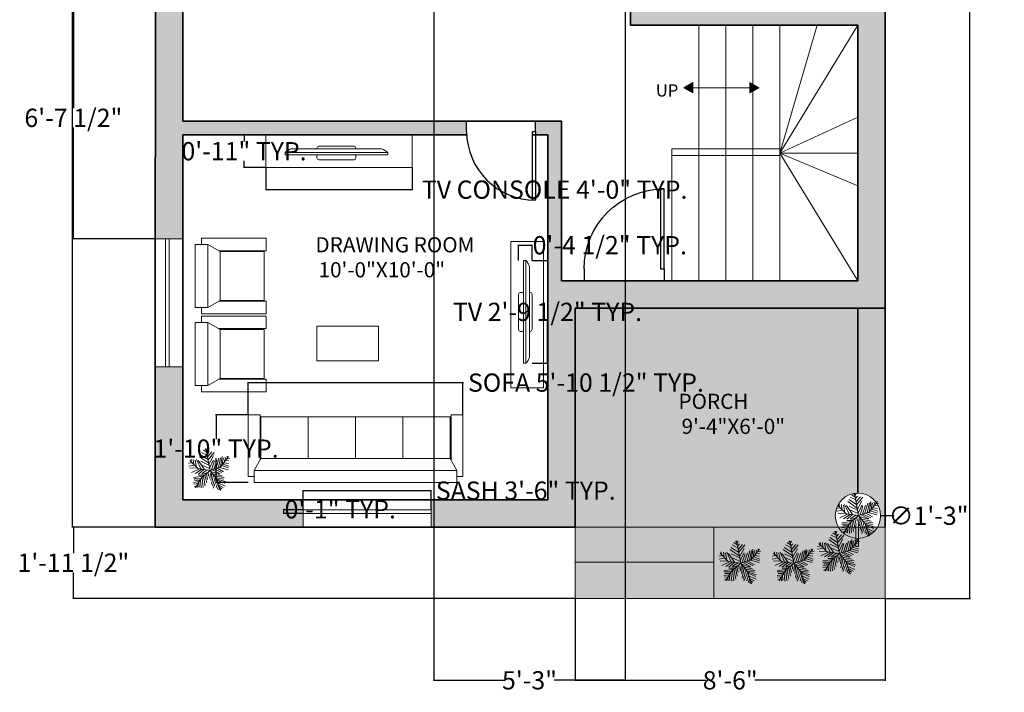
# Model space of a CAD drawing. Units: inches. Extents: x 143233372 to 143233714, y 112671713 to 112672292.
# Tile 1 of 7: x 143233372 to 143233695, y 112671713 to 112671935. Entities that reach past the tile are written whole.
import ezdxf

# ---------------------------------------------------------------- set-up
doc = ezdxf.new("R2010")
doc.units = ezdxf.units.IN
doc.header["$MEASUREMENT"] = 0
doc.layers.get('0').update_dxf_attribs({"color": 104})
for name, color, linetype, lineweight in [('A-ANNO-DIMS', 2, 'Continuous', 18), ('A-ANNO-SYMB', 7, 'Continuous', 18), ('A-AREA-IDEN', 7, 'Continuous', 18), ('A-EQPM', 8, 'Continuous', 18), ('A-FLOR-STRS', 7, 'Continuous', 18), ('doors', 32, 'Continuous', 25), ('furniture', 23, 'Continuous', 18), ('L-PLNT', 92, 'Continuous', 13), ('L-PLNT-BEDS', 94, 'Continuous', 18), ('L-PLNT-PATT', 92, 'Continuous', 9), ('text', 7, 'Continuous', 18), ('walls', 7, 'Continuous', 35), ('windows', 4, 'Continuous', 18)]:
    doc.layers.add(name, color=color, linetype=linetype, lineweight=lineweight)
doc.layers.add('A-FLOR-PATT', color=9, linetype='Continuous', lineweight=9, true_color=0xc7c8ca)
doc.layers.add('A-WALL-PATT', color=18, linetype='Continuous', lineweight=9, true_color=0x000000)
doc.styles.get("Standard").update_dxf_attribs({"font": 'arial.ttf'})
doc.dimstyles.get("Standard").update_dxf_attribs({"dimtxt": 6, "dimasz": 0.18, "dimexe": 0.18, "dimexo": 0.0625, "dimgap": 0.09, "dimtad": 0, "dimtih": 1, "dimtoh": 1, "dimzin": 0, "dimdsep": 46, "dimlunit": 3, "dimtxsty": 'Standard', "dimcen": 0.09, "dimadec": 0, "dimazin": 0, "dimtfac": 1, "dimtofl": 0, "dimtmove": 0, "dimatfit": 3, "dimfxl": 1, "dimtolj": 1, "dimtzin": 0, "dimarcsym": 0})

# ---------------------------------------------------------------- blocks, each defined once
blk = doc.blocks.new('FABRIC SOFA 4S')
at = {"layer": 'furniture'}
for p, q in [((0, -51), (0, 51)), ((6, 51), (0, 51)), ((3, 54), (34, 54)), ((3, 51), (3, 54)), ((6, -51), (6, 51)), ((12, 47.63), (6, 51)), ((34, 48), (34, 54)), ((11.14, 48), (34, 48)), ((33, 23.81), (12, 23.81)), ((33, 0), (12, 0)), ((33, -23.81), (12, -23.81)), ((6, -51), (12, -47.63)), ((11.54, -48), (34, -48)), ((34, -48), (34, -54)), ((6, -51), (0, -51)), ((3, -54), (3, -51)), ((3, -54), (34, -54))]:
    blk.add_line(p, q, dxfattribs=at)
blk.add_lwpolyline([(12, -47.63), (12, 47.63), (33, 47.63), (33, -47.63)], close=True, dxfattribs=at)
blk = doc.blocks.new('FABRIC SOFA 1S')
at = {"layer": 'furniture'}
for p, q in [((0, -15.12), (0, 15.12)), ((6, 15.12), (0, 15.12)), ((3, 18.12), (34, 18.12)), ((3, 15.12), (3, 18.12)), ((6, -15.12), (6, 15.12)), ((12, 11.75), (6, 15.12)), ((34, 12.12), (34, 18.12)), ((11.33, 12.12), (34, 12.12)), ((6, -15.12), (12, -11.75)), ((11.33, -12.12), (34, -12.12)), ((34, -12.12), (34, -18.12)), ((6, -15.12), (0, -15.12)), ((3, -18.12), (3, -15.12)), ((3, -18.12), (34, -18.12))]:
    blk.add_line(p, q, dxfattribs=at)
blk.add_lwpolyline([(12, -11.75), (12, 11.75), (33, 11.75), (33, -11.75)], close=True, dxfattribs=at)
blk = doc.blocks.new('PLASMA-LARGE')
at = {"layer": 'furniture'}
for p, q in [((-7.26, 0), (7.26, 0)), ((-21, -2.5), (21, -2.5)), ((-21, -2.5), (-21, -3.5)), ((-21, -3.5), (21, -3.5)), ((-18.61, -1), (18.61, -1)), ((-8, -1), (-8, -0.74)), ((-8, -3.5), (-8, -4.76)), ((8, -1), (8, -0.74)), ((8, -3.5), (8, -4.76)), ((21, -2.5), (21, -3.5)), ((-7.26, -5.5), (7.26, -5.5))]:
    blk.add_line(p, q, dxfattribs=at)
for centre, radius, start, end in [((-7.26, -0.74), 0.744, 90, 180), ((7.26, -0.74), 0.744, 0, 90), ((-13.97, -11.05), 11.07, 114.7602, 129.4175), ((13.97, -11.05), 11.07, 50.5825, 65.2398), ((-7.26, -4.76), 0.744, 180, 270), ((7.26, -4.76), 0.744, 270, 0)]:
    blk.add_arc(centre, radius, start, end, dxfattribs=at)
blk = doc.blocks.new('*U24')
for p, q in [((0, 0), (0, -6)), ((40, 0), (40, -6))]:
    blk.add_line(p, q)
blk.add_lwpolyline([(0, 0), (0, 40), (1.75, 40), (1.75, 0)], close=True)
blk.add_arc((0, 0), 40, 0, 90)
blk = doc.blocks.new('*U26')
for p, q in [((-8.737, 47.138), (-17.069, 52.711)), ((-10.186, 53.64), (-13.084, 55.962)), ((0, 0), (-10.5, 57)), ((-9.099, 51.782), (-6.563, 55.962)), ((-31.5, 4.5), (-52.5, 25.5)), ((-48.585, 21.131), (-49.309, 29.026)), ((-43.513, 28.561), (-42.427, 15.558)), ((-38.442, 26.239), (-34.819, 7.663)), ((-35.544, 28.097), (-24.314, 3.947)), ((-14.533, 2.09), (-30.834, 25.31)), ((-3.665, 19.273), (-27.574, 35.527)), ((-5.114, 28.097), (-24.676, 40.636)), ((-7.288, 39.707), (-21.778, 46.673)), ((-7.65, 43.423), (-2.578, 49.46)), ((-5.839, 35.992), (4.667, 48.067)), ((-5.114, 27.632), (10.463, 46.673)), ((-2.941, 16.486), (8.652, 37.85)), ((-1.129, 6.734), (9.014, 26.704)), ((10.101, 3.483), (17.708, 26.239)), ((16.259, 5.805), (23.142, 31.348)), ((22.055, 7.198), (27.489, 32.277)), ((27, 9), (48, 36)), ((27.127, 9.056), (31.112, 35.992)), ((31.836, 30.883), (32.561, 16.486)), ((35.096, 32.741), (37.27, 22.524)), ((38.719, 34.134), (41.979, 28.561)), ((40.53, 25.775), (48.862, 24.846)), ((43.791, 29.954), (51.036, 30.883)), ((44.153, 36.456), (45.239, 32.741)), ((-47.498, 19.737), (-55.83, 18.344)), ((-40.615, 13.7), (-55.105, 10.913)), ((-33.37, 6.269), (-52.207, 5.34)), ((-28.299, 3.483), (-47.86, -5.805)), ((-21.416, 3.018), (-38.079, -8.128)), ((0, 0), (-31.5, 4.5)), ((-15.982, 2.09), (-30.11, -9.521)), ((-24.314, 23.917), (-2.941, 13.7)), ((0, 0), (-22.5, -19.5)), ((-6.563, 1.161), (-21.416, -8.128)), ((-20.691, 13.7), (-1.129, 4.876)), ((0, 0), (27, 9)), ((0, 0), (18, -22.5)), ((3.942, 1.625), (11.187, 24.381)), ((6.478, 1.625), (26.04, -8.592)), ((11.187, 3.483), (30.749, -5.805)), ((18.07, 5.805), (35.096, -3.483)), ((24.229, 7.663), (46.688, 1.625)), ((29.662, 12.307), (48.137, 6.269)), ((33.285, 16.486), (48.862, 10.913)), ((36.183, 19.737), (48.137, 17.88)), ((-17.431, -15.094), (-42.789, -18.809)), ((-24.314, -21.596), (-42.427, -22.06)), ((-22.5, -19.5), (-37.5, -45)), ((-15.257, -12.772), (-30.11, -12.772)), ((-25.038, -23.918), (-22.865, -45.281)), ((-20.691, -18.345), (-17.793, -44.352)), ((-6.563, -5.805), (-19.967, -9.985)), ((-17.069, -15.094), (-12.721, -40.172)), ((-13.446, -11.378), (-8.737, -32.741)), ((-9.461, -8.592), (-6.201, -23.453)), ((-4.752, -3.483), (-3.665, -14.629)), ((2.493, -3.019), (-1.491, -20.202)), ((1.769, -2.555), (24.229, -9.521)), ((5.029, -6.27), (2.131, -25.775)), ((9.014, -11.378), (3.58, -35.992)), ((14.085, -16.951), (6.478, -40.172)), ((7.565, -9.056), (32.198, -14.629)), ((18.07, -22.524), (8.289, -45.745)), ((12.274, -15.094), (36.907, -18.809)), ((16.259, -19.738), (36.183, -22.989)), ((18, -22.5), (27, -52.5)), ((18.433, -22.524), (40.53, -29.026)), ((-28.299, -29.026), (-42.789, -31.348)), ((-30.834, -34.135), (-42.427, -35.528)), ((-34.457, -39.708), (-40.978, -42.494)), ((-26.849, -26.24), (-40.253, -25.775)), ((-32.646, -36.921), (-31.921, -44.352)), ((-29.023, -30.884), (-27.936, -43.887)), ((20.244, -30.419), (15.897, -44.816)), ((19.157, -25.311), (38.719, -33.206)), ((22.78, -37.85), (19.519, -48.532)), ((21.331, -32.741), (39.081, -40.636)), ((22.78, -38.314), (34.372, -44.816)), ((24.591, -45.745), (23.142, -50.854)), ((24.591, -43.423), (30.749, -47.603)), ((26.764, -49.925), (28.213, -50.854))]:
    blk.add_line(p, q)
blk = doc.blocks.new('*D28')
at = {"layer": 'A-ANNO-DIMS', "color": 0, "lineweight": -2, "transparency": 16777216}
for p, q in [((143233416.22, 112672249.18), (143233388.75, 112672249.18)), ((143233388.93, 112672249), (143233388.93, 112672011.59)), ((143233388.93, 112671767.86), (143233388.93, 112672005.28)), ((143233416.22, 112671767.68), (143233388.75, 112671767.68))]:
    blk.add_line(p, q, dxfattribs=at)
at = {"layer": 'A-ANNO-DIMS', "color": 0, "transparency": 16777216}
for points in [[(143233388.9, 112672249), (143233388.96, 112672249), (143233388.93, 112672249.18)], [(143233388.9, 112671767.86), (143233388.96, 112671767.86), (143233388.93, 112671767.68)]]:
    blk.add_solid(points, dxfattribs=at)
at = {"layer": 'Defpoints', "color": 0, "transparency": 16777216}
for p in [(143233416.28, 112672249.18), (143233388.93, 112671767.68), (143233416.28, 112671767.68)]:
    blk.add_point(p, dxfattribs=at)
at = {"layer": 'A-ANNO-DIMS', "color": 0, "transparency": 16777216, "insert": (143233388.93, 112672008.43), "char_height": 6, "attachment_point": 5}
blk.add_mtext('\\A1;30\'-0"', dxfattribs=at)
blk = doc.blocks.new('SASH-42IN')
for p, q in [((0, 1.17), (42.12, 1.17)), ((42.12, 0), (0, 0)), ((42.12, 1.17), (42.12, 0))]:
    blk.add_line(p, q)
blk = doc.blocks.new('MEDIA-CONSOLE')
for p, q in [((0, 48.12), (10.82, 48.12)), ((0, 0), (0, 48.12)), ((10.82, 48.12), (10.82, 0)), ((10.82, 0), (0, 0))]:
    blk.add_line(p, q)
blk = doc.blocks.new('*D33')
at = {"layer": 'A-ANNO-DIMS', "color": 0, "lineweight": -2, "transparency": 16777216}
for p, q in [((143233464.81, 112671773.41), (143233464.81, 112671779.85)), ((143233464.99, 112671779.67), (143233506.74, 112671779.67)), ((143233506.92, 112671773.41), (143233506.92, 112671779.85)), ((143233506.92, 112671779.67), (143233507.1, 112671779.67))]:
    blk.add_line(p, q, dxfattribs=at)
at = {"layer": 'A-ANNO-DIMS', "color": 0, "transparency": 16777216}
for points in [[(143233464.99, 112671779.7), (143233464.99, 112671779.64), (143233464.81, 112671779.67)], [(143233506.74, 112671779.7), (143233506.74, 112671779.64), (143233506.92, 112671779.67)]]:
    blk.add_solid(points, dxfattribs=at)
at = {"layer": 'Defpoints', "color": 0, "transparency": 16777216}
for p in [(143233506.92, 112671779.67), (143233464.81, 112671773.35), (143233506.92, 112671773.35)]:
    blk.add_point(p, dxfattribs=at)
at = {"layer": 'A-ANNO-DIMS', "color": 0, "transparency": 16777216, "insert": (143233538.04, 112671779.67), "char_height": 6, "attachment_point": 5}
blk.add_mtext('\\A1;SASH 3\'-6" TYP.', dxfattribs=at)
blk = doc.blocks.new('*D34')
at = {"layer": 'A-ANNO-DIMS', "color": 0, "lineweight": -2, "transparency": 16777216}
for p, q in [((143233464.74, 112671773.35), (143233458.31, 112671773.35)), ((143233464.74, 112671772.18), (143233458.31, 112671772.18)), ((143233458.49, 112671773.35), (143233458.49, 112671773.53)), ((143233458.49, 112671773.53), (143233458.67, 112671773.53)), ((143233458.49, 112671772.36), (143233458.49, 112671773.17))]:
    blk.add_line(p, q, dxfattribs=at)
at = {"layer": 'A-ANNO-DIMS', "color": 0, "transparency": 16777216}
for points in [[(143233458.46, 112671773.17), (143233458.52, 112671773.17), (143233458.49, 112671773.35)], [(143233458.46, 112671772.36), (143233458.52, 112671772.36), (143233458.49, 112671772.18)]]:
    blk.add_solid(points, dxfattribs=at)
at = {"layer": 'Defpoints', "color": 0, "transparency": 16777216}
for p in [(143233458.49, 112671773.35), (143233464.81, 112671773.35), (143233464.81, 112671772.18)]:
    blk.add_point(p, dxfattribs=at)
at = {"layer": 'A-ANNO-DIMS', "color": 0, "transparency": 16777216, "insert": (143233477.04, 112671773.53), "char_height": 6, "attachment_point": 5}
blk.add_mtext('\\A1;0\'-1" TYP.', dxfattribs=at)
blk = doc.blocks.new('*D37')
at = {"layer": 'A-ANNO-DIMS', "color": 0, "lineweight": -2, "transparency": 16777216}
for p, q in [((143233540.19, 112671855.3), (143233545.37, 112671855.3)), ((143233545.19, 112671855.12), (143233545.19, 112671841.63)), ((143233545.19, 112671821.75), (143233545.19, 112671835.24)), ((143233540.19, 112671821.57), (143233545.37, 112671821.57))]:
    blk.add_line(p, q, dxfattribs=at)
at = {"layer": 'A-ANNO-DIMS', "color": 0, "transparency": 16777216}
for points in [[(143233545.16, 112671855.12), (143233545.22, 112671855.12), (143233545.19, 112671855.3)], [(143233545.16, 112671821.75), (143233545.22, 112671821.75), (143233545.19, 112671821.57)]]:
    blk.add_solid(points, dxfattribs=at)
at = {"layer": 'Defpoints', "color": 0, "transparency": 16777216}
for p in [(143233540.13, 112671855.3), (143233540.13, 112671821.57), (143233545.19, 112671821.57)]:
    blk.add_point(p, dxfattribs=at)
at = {"layer": 'A-ANNO-DIMS', "color": 0, "transparency": 16777216, "insert": (143233545.19, 112671838.44), "char_height": 6, "attachment_point": 5}
blk.add_mtext('\\A1;TV 2\'-9 1/2" TYP.', dxfattribs=at)
blk = doc.blocks.new('*D38')
at = {"layer": 'A-ANNO-DIMS', "color": 0, "lineweight": -2, "transparency": 16777216}
for p, q in [((143233535.71, 112671855.36), (143233535.71, 112671860.54)), ((143233535.89, 112671860.36), (143233539.95, 112671860.36)), ((143233540.13, 112671855.36), (143233540.13, 112671860.54)), ((143233540.13, 112671860.36), (143233540.31, 112671860.36))]:
    blk.add_line(p, q, dxfattribs=at)
at = {"layer": 'A-ANNO-DIMS', "color": 0, "transparency": 16777216}
for points in [[(143233535.89, 112671860.39), (143233535.89, 112671860.33), (143233535.71, 112671860.36)], [(143233539.95, 112671860.39), (143233539.95, 112671860.33), (143233540.13, 112671860.36)]]:
    blk.add_solid(points, dxfattribs=at)
at = {"layer": 'Defpoints', "color": 0, "transparency": 16777216}
for p in [(143233540.13, 112671860.36), (143233535.71, 112671855.3), (143233540.13, 112671855.3)]:
    blk.add_point(p, dxfattribs=at)
at = {"layer": 'A-ANNO-DIMS', "color": 0, "transparency": 16777216, "insert": (143233565.68, 112671860.36), "char_height": 6, "attachment_point": 5}
blk.add_mtext('\\A1;0\'-4 1/2" TYP.', dxfattribs=at)
blk = doc.blocks.new('*D39')
at = {"layer": 'A-ANNO-DIMS', "color": 0, "lineweight": -2, "transparency": 16777216}
for p, q in [((143233452.61, 112671885.8), (143233452.61, 112671878.46)), ((143233500.73, 112671885.8), (143233500.73, 112671878.46)), ((143233452.79, 112671878.64), (143233500.55, 112671878.64)), ((143233500.73, 112671878.64), (143233500.91, 112671878.64))]:
    blk.add_line(p, q, dxfattribs=at)
at = {"layer": 'A-ANNO-DIMS', "color": 0, "transparency": 16777216}
for points in [[(143233452.79, 112671878.67), (143233452.79, 112671878.61), (143233452.61, 112671878.64)], [(143233500.55, 112671878.67), (143233500.55, 112671878.61), (143233500.73, 112671878.64)]]:
    blk.add_solid(points, dxfattribs=at)
at = {"layer": 'Defpoints', "color": 0, "transparency": 16777216}
for p in [(143233452.61, 112671885.86), (143233500.73, 112671885.86), (143233500.73, 112671878.64)]:
    blk.add_point(p, dxfattribs=at)
at = {"layer": 'A-ANNO-DIMS', "color": 0, "transparency": 16777216, "insert": (143233547.54, 112671878.64), "char_height": 6, "attachment_point": 5}
blk.add_mtext('\\A1;TV CONSOLE 4\'-0" TYP.', dxfattribs=at)
blk = doc.blocks.new('*D40')
at = {"layer": 'A-ANNO-DIMS', "color": 0, "lineweight": -2, "transparency": 16777216}
for p, q in [((143233452.55, 112671896.68), (143233445.21, 112671896.68)), ((143233445.39, 112671896.5), (143233445.39, 112671894.42)), ((143233445.39, 112671886.04), (143233445.39, 112671888.12)), ((143233452.55, 112671885.86), (143233445.21, 112671885.86))]:
    blk.add_line(p, q, dxfattribs=at)
at = {"layer": 'A-ANNO-DIMS', "color": 0, "transparency": 16777216}
for points in [[(143233445.36, 112671896.5), (143233445.42, 112671896.5), (143233445.39, 112671896.68)], [(143233445.36, 112671886.04), (143233445.42, 112671886.04), (143233445.39, 112671885.86)]]:
    blk.add_solid(points, dxfattribs=at)
at = {"layer": 'Defpoints', "color": 0, "transparency": 16777216}
for p in [(143233452.61, 112671896.68), (143233445.39, 112671885.86), (143233452.61, 112671885.86)]:
    blk.add_point(p, dxfattribs=at)
at = {"layer": 'A-ANNO-DIMS', "color": 0, "transparency": 16777216, "insert": (143233445.39, 112671891.27), "char_height": 6, "attachment_point": 5}
blk.add_mtext('\\A1;0\'-11" TYP.', dxfattribs=at)
blk = doc.blocks.new('*D45')
at = {"layer": 'A-ANNO-DIMS', "color": 0, "lineweight": -2, "transparency": 16777216}
for p, q in [((143233446.78, 112671804.66), (143233446.78, 112671815.37)), ((143233446.96, 112671815.19), (143233517.21, 112671815.19)), ((143233517.39, 112671804.66), (143233517.39, 112671815.37)), ((143233517.39, 112671815.19), (143233517.57, 112671815.19))]:
    blk.add_line(p, q, dxfattribs=at)
at = {"layer": 'A-ANNO-DIMS', "color": 0, "transparency": 16777216}
for points in [[(143233446.96, 112671815.22), (143233446.96, 112671815.16), (143233446.78, 112671815.19)], [(143233517.21, 112671815.22), (143233517.21, 112671815.16), (143233517.39, 112671815.19)]]:
    blk.add_solid(points, dxfattribs=at)
at = {"layer": 'Defpoints', "color": 0, "transparency": 16777216}
for p in [(143233517.39, 112671815.19), (143233446.78, 112671804.6), (143233517.39, 112671804.6)]:
    blk.add_point(p, dxfattribs=at)
at = {"layer": 'A-ANNO-DIMS', "color": 0, "transparency": 16777216, "insert": (143233557.83, 112671815.19), "char_height": 6, "attachment_point": 5}
blk.add_mtext('\\A1;SOFA 5\'-10 1/2" TYP.', dxfattribs=at)
blk = doc.blocks.new('*D46')
at = {"layer": 'A-ANNO-DIMS', "color": 0, "lineweight": -2, "transparency": 16777216}
for p, q in [((143233446.71, 112671804.6), (143233436.01, 112671804.6)), ((143233436.19, 112671804.42), (143233436.19, 112671796.64)), ((143233436.19, 112671782.55), (143233436.19, 112671790.33)), ((143233446.71, 112671782.37), (143233436.01, 112671782.37))]:
    blk.add_line(p, q, dxfattribs=at)
at = {"layer": 'A-ANNO-DIMS', "color": 0, "transparency": 16777216}
for points in [[(143233436.16, 112671804.42), (143233436.22, 112671804.42), (143233436.19, 112671804.6)], [(143233436.16, 112671782.55), (143233436.22, 112671782.55), (143233436.19, 112671782.37)]]:
    blk.add_solid(points, dxfattribs=at)
at = {"layer": 'Defpoints', "color": 0, "transparency": 16777216}
for p in [(143233436.19, 112671804.6), (143233446.78, 112671804.6), (143233446.78, 112671782.37)]:
    blk.add_point(p, dxfattribs=at)
at = {"layer": 'A-ANNO-DIMS', "color": 0, "transparency": 16777216, "insert": (143233436.19, 112671793.49), "char_height": 6, "attachment_point": 5}
blk.add_mtext('\\A1;1\'-10" TYP.', dxfattribs=at)
blk = doc.blocks.new('*D63')
at = {"layer": 'A-ANNO-DIMS', "color": 0, "lineweight": -2, "transparency": 16777216}
for p, q in [((143233656.35, 112672249.18), (143233684.29, 112672249.18)), ((143233684.11, 112672249), (143233684.11, 112671999.82)), ((143233684.11, 112671744.43), (143233684.11, 112671993.61)), ((143233656.35, 112671744.25), (143233684.29, 112671744.25))]:
    blk.add_line(p, q, dxfattribs=at)
at = {"layer": 'A-ANNO-DIMS', "color": 0, "transparency": 16777216}
for points in [[(143233684.08, 112672249), (143233684.14, 112672249), (143233684.11, 112672249.18)], [(143233684.08, 112671744.43), (143233684.14, 112671744.43), (143233684.11, 112671744.25)]]:
    blk.add_solid(points, dxfattribs=at)
at = {"layer": 'Defpoints', "color": 0, "transparency": 16777216}
for p in [(143233656.28, 112672249.18), (143233656.28, 112671744.25), (143233684.11, 112671744.25)]:
    blk.add_point(p, dxfattribs=at)
at = {"layer": 'A-ANNO-DIMS', "color": 0, "transparency": 16777216, "insert": (143233684.11, 112671996.72), "char_height": 6, "attachment_point": 5}
blk.add_mtext('\\A1;42\'-1"', dxfattribs=at)
blk = doc.blocks.new('*D67')
at = {"layer": 'A-ANNO-DIMS', "color": 0, "lineweight": -2, "transparency": 16777216}
for p, q in [((143233554.28, 112671744.19), (143233554.28, 112671717.12)), ((143233656.28, 112671744.19), (143233656.28, 112671717.12)), ((143233554.46, 112671717.3), (143233597.22, 112671717.3)), ((143233656.1, 112671717.3), (143233613.35, 112671717.3))]:
    blk.add_line(p, q, dxfattribs=at)
at = {"layer": 'A-ANNO-DIMS', "color": 0, "transparency": 16777216}
for points in [[(143233554.46, 112671717.33), (143233554.46, 112671717.27), (143233554.28, 112671717.3)], [(143233656.1, 112671717.33), (143233656.1, 112671717.27), (143233656.28, 112671717.3)]]:
    blk.add_solid(points, dxfattribs=at)
at = {"layer": 'Defpoints', "color": 0, "transparency": 16777216}
for p in [(143233554.28, 112671744.25), (143233656.28, 112671744.25), (143233554.28, 112671717.3)]:
    blk.add_point(p, dxfattribs=at)
at = {"layer": 'A-ANNO-DIMS', "color": 0, "transparency": 16777216, "insert": (143233605.28, 112671717.3), "char_height": 6, "attachment_point": 5}
blk.add_mtext('\\A1;8\'-6"', dxfattribs=at)
blk = doc.blocks.new('*D68')
at = {"layer": 'A-ANNO-DIMS', "color": 0, "lineweight": -2, "transparency": 16777216}
for p, q in [((143233554.22, 112671767.68), (143233389.09, 112671767.68)), ((143233389.27, 112671767.5), (143233389.27, 112671759.16)), ((143233389.27, 112671744.43), (143233389.27, 112671752.77)), ((143233554.22, 112671744.25), (143233389.09, 112671744.25))]:
    blk.add_line(p, q, dxfattribs=at)
at = {"layer": 'A-ANNO-DIMS', "color": 0, "transparency": 16777216}
for points in [[(143233389.24, 112671767.5), (143233389.3, 112671767.5), (143233389.27, 112671767.68)], [(143233389.24, 112671744.43), (143233389.3, 112671744.43), (143233389.27, 112671744.25)]]:
    blk.add_solid(points, dxfattribs=at)
at = {"layer": 'Defpoints', "color": 0, "transparency": 16777216}
for p in [(143233389.27, 112671767.68), (143233554.28, 112671767.68), (143233554.28, 112671744.25)]:
    blk.add_point(p, dxfattribs=at)
at = {"layer": 'A-ANNO-DIMS', "color": 0, "transparency": 16777216, "insert": (143233389.27, 112671755.97), "char_height": 6, "attachment_point": 5}
blk.add_mtext('\\A1;1\'-11 1/2"', dxfattribs=at)
blk = doc.blocks.new('*D69')
at = {"layer": 'A-ANNO-DIMS', "color": 0, "lineweight": -2, "transparency": 16777216}
for p, q in [((143233507.78, 112672033.12), (143233507.78, 112671717.12)), ((143233570.78, 112672033.12), (143233570.78, 112671717.12)), ((143233507.96, 112671717.3), (143233531.22, 112671717.3)), ((143233570.6, 112671717.3), (143233547.35, 112671717.3))]:
    blk.add_line(p, q, dxfattribs=at)
at = {"layer": 'A-ANNO-DIMS', "color": 0, "transparency": 16777216}
for points in [[(143233507.96, 112671717.33), (143233507.96, 112671717.27), (143233507.78, 112671717.3)], [(143233570.6, 112671717.33), (143233570.6, 112671717.27), (143233570.78, 112671717.3)]]:
    blk.add_solid(points, dxfattribs=at)
at = {"layer": 'Defpoints', "color": 0, "transparency": 16777216}
for p in [(143233507.78, 112672033.18), (143233570.78, 112672033.18), (143233570.78, 112671717.3)]:
    blk.add_point(p, dxfattribs=at)
at = {"layer": 'A-ANNO-DIMS', "color": 0, "transparency": 16777216, "insert": (143233539.28, 112671717.3), "char_height": 6, "attachment_point": 5}
blk.add_mtext('\\A1;5\'-3"', dxfattribs=at)
blk = doc.blocks.new('*D73')
at = {"layer": 'A-ANNO-DIMS', "color": 0, "lineweight": -2, "transparency": 16777216}
for p, q in [((143233416.22, 112671942.04), (143233389.09, 112671942.04)), ((143233389.27, 112671941.86), (143233389.27, 112671905.44)), ((143233389.27, 112671862.63), (143233389.27, 112671899.05)), ((143233416.22, 112671862.45), (143233389.09, 112671862.45))]:
    blk.add_line(p, q, dxfattribs=at)
at = {"layer": 'A-ANNO-DIMS', "color": 0, "transparency": 16777216}
for points in [[(143233389.24, 112671941.86), (143233389.3, 112671941.86), (143233389.27, 112671942.04)], [(143233389.24, 112671862.63), (143233389.3, 112671862.63), (143233389.27, 112671862.45)]]:
    blk.add_solid(points, dxfattribs=at)
at = {"layer": 'Defpoints', "color": 0, "transparency": 16777216}
for p in [(143233389.27, 112671942.04), (143233416.28, 112671942.04), (143233416.28, 112671862.45)]:
    blk.add_point(p, dxfattribs=at)
at = {"layer": 'A-ANNO-DIMS', "color": 0, "transparency": 16777216, "insert": (143233389.27, 112671902.24), "char_height": 6, "attachment_point": 5}
blk.add_mtext('\\A1;6\'-7 1/2"', dxfattribs=at)
blk = doc.blocks.new('*D78')
at = {"layer": 'A-ANNO-DIMS', "color": 0, "lineweight": -2, "transparency": 16777216}
for p, q in [((143233647.19, 112671771.42), (143233647.37, 112671771.42)), ((143233647.28, 112671771.33), (143233647.28, 112671771.51)), ((143233659.18, 112671771.42), (143233654.9, 112671771.42))]:
    blk.add_line(p, q, dxfattribs=at)
at = {"layer": 'A-ANNO-DIMS', "color": 0, "transparency": 16777216}
blk.add_solid([(143233654.9, 112671771.45), (143233654.9, 112671771.39), (143233654.72, 112671771.42)], dxfattribs=at)
at = {"layer": 'Defpoints', "color": 0, "transparency": 16777216}
for p in [(143233639.85, 112671771.42), (143233654.72, 112671771.42)]:
    blk.add_point(p, dxfattribs=at)
at = {"layer": 'A-ANNO-DIMS', "color": 0, "transparency": 16777216, "insert": (143233670.51, 112671771.42), "char_height": 6, "attachment_point": 5}
blk.add_mtext('\\A1;∅1\'-3"', dxfattribs=at)

msp = doc.modelspace()

# ---------------------------------------------------------------- hatches: boundary and pattern name
at = {"layer": 'A-ANNO-SYMB'}
h = msp.add_hatch(color=256, dxfattribs=at)
h.dxf.hatch_style = 1
h.paths.add_polyline_path([(143233593.014, 112671913.81), (143233589.979, 112671912.056), (143233593.014, 112671910.417)])
h = msp.add_hatch(color=256, dxfattribs=at)
h.dxf.hatch_style = 1
h.paths.add_polyline_path([(143233611.75, 112671910.417), (143233614.785, 112671912.056), (143233611.75, 112671913.81)])
at = {"layer": 'A-FLOR-PATT'}
h = msp.add_hatch(color=256, dxfattribs=at)
h.dxf.hatch_style = 1
h.paths.add_polyline_path([(143233647.285, 112671839.682), (143233554.285, 112671839.682), (143233554.285, 112671767.682), (143233599.887, 112671767.682), (143233640.858, 112671767.682, -0.1325091), (143233639.849, 112671771.421, -0.4142136), (143233647.285, 112671778.857)])
h.paths.add_polyline_path([(143233656.285, 112671839.682), (143233647.285, 112671839.682), (143233647.285, 112671778.857, -0.4142136), (143233654.72, 112671771.421, -0.1325091), (143233653.711, 112671767.682), (143233656.285, 112671767.682)])
h.paths.add_polyline_path([(143233599.887, 112671767.682), (143233599.887, 112671767.682), (143233554.285, 112671767.682), (143233554.285, 112671756.172), (143233599.887, 112671756.172)])
h.paths.add_polyline_path([(143233599.887, 112671756.172), (143233554.285, 112671756.172), (143233554.285, 112671744.249), (143233599.887, 112671744.249)])
at = {"layer": 'A-WALL-PATT'}
h = msp.add_hatch(color=256, dxfattribs=at)
h.dxf.hatch_style = 1
h.paths.add_polyline_path([(143233425.285, 112671820.328), (143233416.222, 112671820.328), (143233416.222, 112671767.682), (143233464.805, 112671767.682), (143233464.805, 112671776.682), (143233425.285, 112671776.682)])
h.paths.add_polyline_path([(143233425.285, 112672055.48), (143233416.285, 112672055.48), (143233416.285, 112671984.159), (143233425.285, 112671984.159)])
h.paths.add_polyline_path([(143233656.285, 112671963.912), (143233647.285, 112671963.912), (143233647.285, 112671848.682), (143233647.285, 112671839.682), (143233656.285, 112671839.682), (143233656.285, 112671889.182)])
h.paths.add_polyline_path([(143233425.285, 112672097.332), (143233425.285, 112672097.332), (143233425.285, 112672108.216), (143233425.285, 112672240.182), (143233451.497, 112672240.182), (143233451.497, 112672249.182), (143233416.285, 112672249.182), (143233416.285, 112672079.453), (143233420.069, 112672079.453), (143233425.285, 112672079.453)])
h.paths.add_polyline_path([(143233576.214, 112672249.182), (143233493.616, 112672249.182), (143233493.616, 112672240.182), (143233576.214, 112672240.182)])
h.paths.add_polyline_path([(143233425.285, 112671942.039), (143233416.285, 112671942.039), (143233416.285, 112671889.182), (143233416.271, 112671862.447), (143233425.285, 112671862.447), (143233425.285, 112671896.682), (143233518.63, 112671896.682, -0.0122006), (143233518.603, 112671897.787), (143233518.603, 112671901.182), (143233425.285, 112671901.182)])
h = msp.add_hatch(color=256, dxfattribs=at)
h.dxf.hatch_style = 1
h.paths.add_polyline_path([(143233549.785, 112671901.182), (143233541.241, 112671901.182), (143233541.241, 112671897.787), (143233541.241, 112671896.682), (143233545.285, 112671896.682), (143233545.285, 112671848.682), (143233549.785, 112671848.682)])
h.paths.add_polyline_path([(143233581.285, 112672033.182), (143233576.785, 112672033.182), (143233576.785, 112672011.912), (143233581.285, 112672011.912)])
h = msp.add_hatch(color=256, dxfattribs=at)
h.dxf.hatch_style = 1
h.paths.add_polyline_path([(143233647.285, 112671937.182), (143233572.511, 112671937.182), (143233572.511, 112671932.682), (143233647.285, 112671932.682)])
h = msp.add_hatch(color=256, dxfattribs=at)
h.dxf.hatch_style = 1
h.paths.add_polyline_path([(143233549.785, 112671848.682), (143233545.285, 112671848.682), (143233545.285, 112671776.682), (143233506.924, 112671776.682), (143233506.924, 112671767.682), (143233549.785, 112671767.682)])
h = msp.add_hatch(color=256, dxfattribs=at)
h.dxf.hatch_style = 1
h.paths.add_polyline_path([(143233647.285, 112671848.682), (143233583.553, 112671848.682), (143233545.285, 112671848.682), (143233545.285, 112671839.682), (143233647.285, 112671839.682)])
h = msp.add_hatch(color=256, dxfattribs=at)
h.dxf.hatch_style = 1
h.paths.add_polyline_path([(143233554.285, 112671839.682), (143233545.285, 112671839.682), (143233545.285, 112671776.682), (143233506.924, 112671776.682), (143233506.924, 112671767.682), (143233549.785, 112671767.682), (143233554.285, 112671767.682)])
at = {"layer": 'L-PLNT-PATT'}
h = msp.add_hatch(color=256, dxfattribs=at)
h.dxf.hatch_style = 1
h.paths.add_polyline_path([(143233656.285, 112671767.682), (143233599.887, 112671767.682), (143233599.887, 112671756.172), (143233599.887, 112671744.249), (143233656.285, 112671744.249)])

# ---------------------------------------------------------------- linework, layer by layer
at = {"layer": 'A-ANNO-SYMB'}
for p, q in [((143233589.979, 112671912.056), (143233593.014, 112671913.81)), ((143233593.014, 112671913.81), (143233593.014, 112671910.417)), ((143233611.75, 112671913.81), (143233611.75, 112671910.417)), ((143233614.785, 112671912.056), (143233611.75, 112671913.81)), ((143233593.014, 112671910.417), (143233589.979, 112671912.056)), ((143233593.014, 112671912.056), (143233614.785, 112671912.056)), ((143233611.75, 112671910.417), (143233614.785, 112671912.056))]:
    msp.add_line(p, q, dxfattribs=at)
at = {"layer": 'A-FLOR-STRS'}
for p, q in [((143233594.938, 112671848.682), (143233594.938, 112671932.682)), ((143233603.831, 112671848.682), (143233603.831, 112671932.682)), ((143233612.724, 112671848.682), (143233612.724, 112671932.682)), ((143233621.617, 112671848.682), (143233621.617, 112671932.682)), ((143233621.617, 112671890.682), (143233647.285, 112671932.682)), ((143233621.617, 112671890.682), (143233633.85, 112671932.682)), ((143233621.617, 112671890.682), (143233647.285, 112671902.483)), ((143233621.617, 112671892.019), (143233586.045, 112671892.019)), ((143233586.045, 112671892.019), (143233586.045, 112671889.902)), ((143233586.045, 112671848.682), (143233586.045, 112671889.902)), ((143233586.045, 112671889.902), (143233621.617, 112671889.902)), ((143233621.617, 112671890.682), (143233647.285, 112671890.682)), ((143233621.617, 112671890.682), (143233647.285, 112671879.905)), ((143233621.617, 112671890.682), (143233647.285, 112671848.682)), ((143233554.285, 112671744.249), (143233554.285, 112671767.682)), ((143233554.285, 112671767.682), (143233599.887, 112671767.682)), ((143233599.887, 112671756.172), (143233599.887, 112671767.682)), ((143233599.887, 112671767.682), (143233599.887, 112671756.172)), ((143233599.887, 112671767.682), (143233599.887, 112671756.172)), ((143233599.887, 112671756.172), (143233554.285, 112671756.172)), ((143233599.887, 112671744.249), (143233554.285, 112671744.249))]:
    msp.add_line(p, q, dxfattribs=at)
at = {"layer": 'furniture'}
for p, q in [((143233489.635, 112671833.691), (143233469.349, 112671833.691)), ((143233469.349, 112671833.691), (143233469.349, 112671822.319)), ((143233489.635, 112671822.319), (143233489.635, 112671833.691)), ((143233469.349, 112671822.319), (143233489.635, 112671822.319))]:
    msp.add_line(p, q, dxfattribs=at)
at = {"layer": 'L-PLNT'}
for p, q in [((143233646.597, 112671768.43), (143233646.597, 112671761.303)), ((143233647.42, 112671761.343), (143233647.42, 112671768.8)), ((143233646.597, 112671761.303), (143233647.42, 112671761.343))]:
    msp.add_line(p, q, dxfattribs=at)
at = {"layer": 'L-PLNT-BEDS'}
for p, q in [((143233599.887, 112671756.172), (143233599.887, 112671767.682)), ((143233599.887, 112671767.682), (143233656.285, 112671767.682)), ((143233656.285, 112671744.249), (143233656.285, 112671767.682)), ((143233599.887, 112671744.249), (143233599.887, 112671756.172)), ((143233599.887, 112671744.249), (143233656.285, 112671744.249))]:
    msp.add_line(p, q, dxfattribs=at)
msp.add_circle((143233647.285, 112671771.421), 7.435, dxfattribs=at)
at = {"layer": 'walls'}
for p, q in [((143233416.285, 112671889.182), (143233416.285, 112672249.182)), ((143233656.285, 112672249.182), (143233656.285, 112671889.182)), ((143233425.285, 112671901.182), (143233425.285, 112672240.182)), ((143233572.511, 112671937.182), (143233572.511, 112671932.682)), ((143233572.511, 112671932.682), (143233647.285, 112671932.682)), ((143233647.285, 112671932.682), (143233647.285, 112671848.682)), ((143233425.285, 112671901.182), (143233549.785, 112671901.182)), ((143233549.785, 112671901.182), (143233549.785, 112671848.682)), ((143233425.285, 112671896.682), (143233518.63, 112671896.682)), ((143233425.285, 112671896.682), (143233425.285, 112671776.682)), ((143233540.251, 112671896.682), (143233545.285, 112671896.682)), ((143233545.285, 112671896.682), (143233545.285, 112671776.682)), ((143233416.222, 112671889.182), (143233416.222, 112671767.682)), ((143233647.285, 112671848.682), (143233647.285, 112671889.182)), ((143233656.285, 112671767.682), (143233656.285, 112671889.182)), ((143233549.785, 112671848.682), (143233586.045, 112671848.682)), ((143233583.553, 112671848.682), (143233647.285, 112671848.682)), ((143233554.285, 112671839.682), (143233656.285, 112671839.682)), ((143233554.285, 112671839.682), (143233554.285, 112671767.682)), ((143233554.285, 112671767.682), (143233554.285, 112671839.682)), ((143233647.285, 112671778.857), (143233647.285, 112671839.682)), ((143233425.285, 112671776.682), (143233545.285, 112671776.682)), ((143233416.222, 112671767.682), (143233549.785, 112671767.682)), ((143233549.785, 112671767.682), (143233554.285, 112671767.682))]:
    msp.add_line(p, q, dxfattribs=at)
at = {"layer": 'windows'}
for p, q in [((143233425.285, 112671862.447), (143233416.285, 112671862.447)), ((143233416.285, 112671820.328), (143233425.285, 112671820.328)), ((143233464.805, 112671776.682), (143233464.805, 112671767.682)), ((143233506.924, 112671767.682), (143233506.924, 112671776.682))]:
    msp.add_line(p, q, dxfattribs=at)

# ---------------------------------------------------------------- block references
at = {"layer": 'A-EQPM', "xscale": 0.8031214548296134, "yscale": 0.8031214548296134, "zscale": 0.8031214548296134}
msp.add_blockref('PLASMA-LARGE', (143233475.771, 112671892.899), dxfattribs=at)
at = {"layer": 'A-EQPM', "xscale": 0.8031214548296134, "yscale": 0.8031214548296134, "zscale": 0.8031214548296134, "rotation": 270}
msp.add_blockref('PLASMA-LARGE', (143233540.129, 112671838.437), dxfattribs=at)
at = {"layer": 'doors', "xscale": 0.5659503506931075, "yscale": 0.5659503506931075, "zscale": 0.5659503506931075, "rotation": 180}
msp.add_blockref('*U24', (143233541.241, 112671897.787), dxfattribs=at)
at = {"layer": 'doors', "xscale": -0.6569374701614324, "yscale": 0.6569374701614324, "zscale": 0.6569374701614324}
msp.add_blockref('*U24', (143233583.553, 112671852.624), dxfattribs=at)
at = {"layer": 'furniture'}
for p, rotation in [((143233452.608, 112671896.682), 270.0000000159984), ((143233543.912, 112671861.6), 180)]:
    msp.add_blockref('MEDIA-CONSOLE', p, dxfattribs=dict(at, rotation=rotation))
at = {"layer": 'furniture', "xscale": 0.685544738852578, "yscale": 0.685544738852578, "zscale": 0.685544738852578}
for p in [(143233429.358, 112671850.229), (143233429.358, 112671824.621)]:
    msp.add_blockref('FABRIC SOFA 1S', p, dxfattribs=at)
at = {"layer": 'furniture', "xscale": -0.6537939928824033, "yscale": 0.6537939928824033, "zscale": 0.6537939928824033, "rotation": 269.9999999998932}
msp.add_blockref('FABRIC SOFA 4S', (143233482.082, 112671782.372), dxfattribs=at)
at = {"layer": 'L-PLNT'}
for p, xscale, yscale, zscale in [((143233434.216, 112671786.331), 0.1267628913715484, 0.1267628913715484, 0.1267628913715484), ((143233647.504, 112671771.469), 0.1291622459209909, 0.1291622459209909, 0.1291622459209909), ((143233641.247, 112671758.976), 0.1291622459209909, 0.1291622459209909, 0.1291622459209909), ((143233608.722, 112671755.777), 0.1291622459209909, 0.1291622459209909, 0.1291622459209909), ((143233626.249, 112671755.777), 0.1291622459209909, 0.1291622459209909, 0.1291622459209909)]:
    msp.add_blockref('*U26', p, dxfattribs=dict(at, xscale=xscale, yscale=yscale, zscale=zscale))
at = {"layer": 'windows', "rotation": 90.00000009117734}
msp.add_blockref('SASH-42IN', (143233420.785, 112671820.328), dxfattribs=at)
at = {"layer": 'windows'}
msp.add_blockref('SASH-42IN', (143233464.806, 112671772.182), dxfattribs=at)

# ---------------------------------------------------------------- texts
at = {"layer": 'A-AREA-IDEN'}
for s, p in [('DRAWING ROOM', (143233468.875, 112671858.003)), ('10\'-0"X10\'-0"', (143233469.892, 112671849.789)), ('PORCH', (143233588.263, 112671806.528)), ('9\'-4"X6\'-0"', (143233589.281, 112671798.314))]:
    msp.add_text(s, height=5, dxfattribs=at).set_placement(p)
at = {"layer": 'text'}
msp.add_text('UP', height=4, dxfattribs=at).set_placement((143233580.821, 112671909.254))

# ---------------------------------------------------------------- dimensions: what is measured, and where the dimension line sits
at = {"layer": 'A-ANNO-DIMS'}
for base, p1, p2, angle, text, override, picture, middle in [((143233388.932, 112671767.682), (143233416.285, 112672249.182), (143233416.285, 112671767.682), 90, '30\'-0"', {"dimclrd": 0, "dimclre": 0, "dimclrt": 0}, '*D28', (143233388.932, 112672008.432)), ((143233445.389, 112671885.86), (143233452.608, 112671896.682), (143233452.608, 112671885.86), 270, '<> TYP.', {"dimdec": 1, "dimlfac": 1, "dimrnd": 0, "dimzin": 1, "dimdsep": 46, "dimlunit": 4, "dimfrac": 2}, '*D40', (143233445.389, 112671891.271)), ((143233500.733, 112671878.641), (143233452.608, 112671885.86), (143233500.733, 112671885.86), 0, 'TV CONSOLE <> TYP.', {"dimdec": 1, "dimlfac": 1, "dimrnd": 0, "dimzin": 1, "dimdsep": 46, "dimlunit": 4, "dimfrac": 2}, '*D39', (143233547.544, 112671878.641)), ((143233545.189, 112671821.571), (143233540.129, 112671855.302), (143233540.129, 112671821.571), 270, 'TV <> TYP.', {"dimdec": 1, "dimlfac": 1, "dimrnd": 0, "dimzin": 1, "dimdsep": 46, "dimlunit": 4, "dimfrac": 2}, '*D37', (143233545.189, 112671838.437)), ((143233436.186, 112671804.601), (143233446.777, 112671782.372), (143233446.777, 112671804.601), 90, '<> TYP.', {"dimdec": 1, "dimlfac": 1, "dimrnd": 0, "dimzin": 1, "dimdsep": 46, "dimlunit": 4, "dimfrac": 2}, '*D46', (143233436.186, 112671793.486)), ((143233458.487, 112671773.352), (143233464.805, 112671772.182), (143233464.805, 112671773.352), 90, '<> TYP.', {"dimdec": 1, "dimlfac": 1, "dimrnd": 0, "dimzin": 1, "dimdsep": 46, "dimlunit": 4, "dimfrac": 2}, '*D34', (143233477.044, 112671773.532))]:
    dim = msp.add_linear_dim(base=base, p1=p1, p2=p2, angle=angle, text=text, dimstyle='Standard', override=override, dxfattribs=at)
    dim.commit()
    dim.dimension.update_dxf_attribs({"geometry": picture, "text_midpoint": middle})
for base, p1, p2, picture, middle in [((143233684.111, 112671744.249), (143233656.285, 112672249.182), (143233656.285, 112671744.249), '*D63', (143233684.111, 112671996.716)), ((143233389.272, 112671942.039), (143233416.285, 112671862.447), (143233416.285, 112671942.039), '*D73', (143233389.272, 112671902.243)), ((143233389.272, 112671767.682), (143233554.285, 112671744.249), (143233554.285, 112671767.682), '*D68', (143233389.272, 112671755.966))]:
    dim = msp.add_linear_dim(base=base, p1=p1, p2=p2, angle=90, dimstyle='Standard', override={"dimdec": 1, "dimlfac": 1, "dimrnd": 0, "dimzin": 1, "dimdsep": 46, "dimlunit": 4, "dimfrac": 2}, dxfattribs=at)
    dim.commit()
    dim.dimension.update_dxf_attribs({"geometry": picture, "text_midpoint": middle})
for base, p1, p2, picture, middle in [((143233570.785, 112671717.299), (143233507.785, 112672033.182), (143233570.785, 112672033.182), '*D69', (143233539.285, 112671717.299)), ((143233554.285, 112671717.299), (143233656.285, 112671744.249), (143233554.285, 112671744.249), '*D67', (143233605.285, 112671717.299))]:
    dim = msp.add_linear_dim(base=base, p1=p1, p2=p2, dimstyle='Standard', override={"dimdec": 1, "dimlfac": 1, "dimrnd": 0, "dimzin": 1, "dimdsep": 46, "dimlunit": 4, "dimfrac": 2}, dxfattribs=at)
    dim.commit()
    dim.dimension.update_dxf_attribs({"geometry": picture, "text_midpoint": middle})
for base, p1, p2, text, picture, middle in [((143233540.129, 112671860.362), (143233535.712, 112671855.302), (143233540.129, 112671855.302), '<> TYP.', '*D38', (143233565.676, 112671860.362)), ((143233517.387, 112671815.192), (143233446.777, 112671804.601), (143233517.387, 112671804.601), 'SOFA <> TYP.', '*D45', (143233557.826, 112671815.192)), ((143233506.924, 112671779.67), (143233464.805, 112671773.352), (143233506.924, 112671773.352), 'SASH <> TYP.', '*D33', (143233538.044, 112671779.67))]:
    dim = msp.add_linear_dim(base=base, p1=p1, p2=p2, text=text, dimstyle='Standard', override={"dimdec": 1, "dimlfac": 1, "dimrnd": 0, "dimzin": 1, "dimdsep": 46, "dimlunit": 4, "dimfrac": 2}, dxfattribs=at)
    dim.commit()
    dim.dimension.update_dxf_attribs({"geometry": picture, "text_midpoint": middle})
dim = msp.add_diameter_dim_2p(p1=(143233639.849, 112671771.422), p2=(143233654.72, 112671771.421), dimstyle='Standard', override={"dimdec": 1, "dimlfac": 1, "dimrnd": 0, "dimzin": 1, "dimdsep": 46, "dimlunit": 4, "dimfrac": 2}, dxfattribs=at)
dim.commit()
dim.dimension.update_dxf_attribs({"geometry": '*D78', "text_midpoint": (143233659.181, 112671771.421), "dimtype": 163})

doc.saveas('drawing.dxf')
